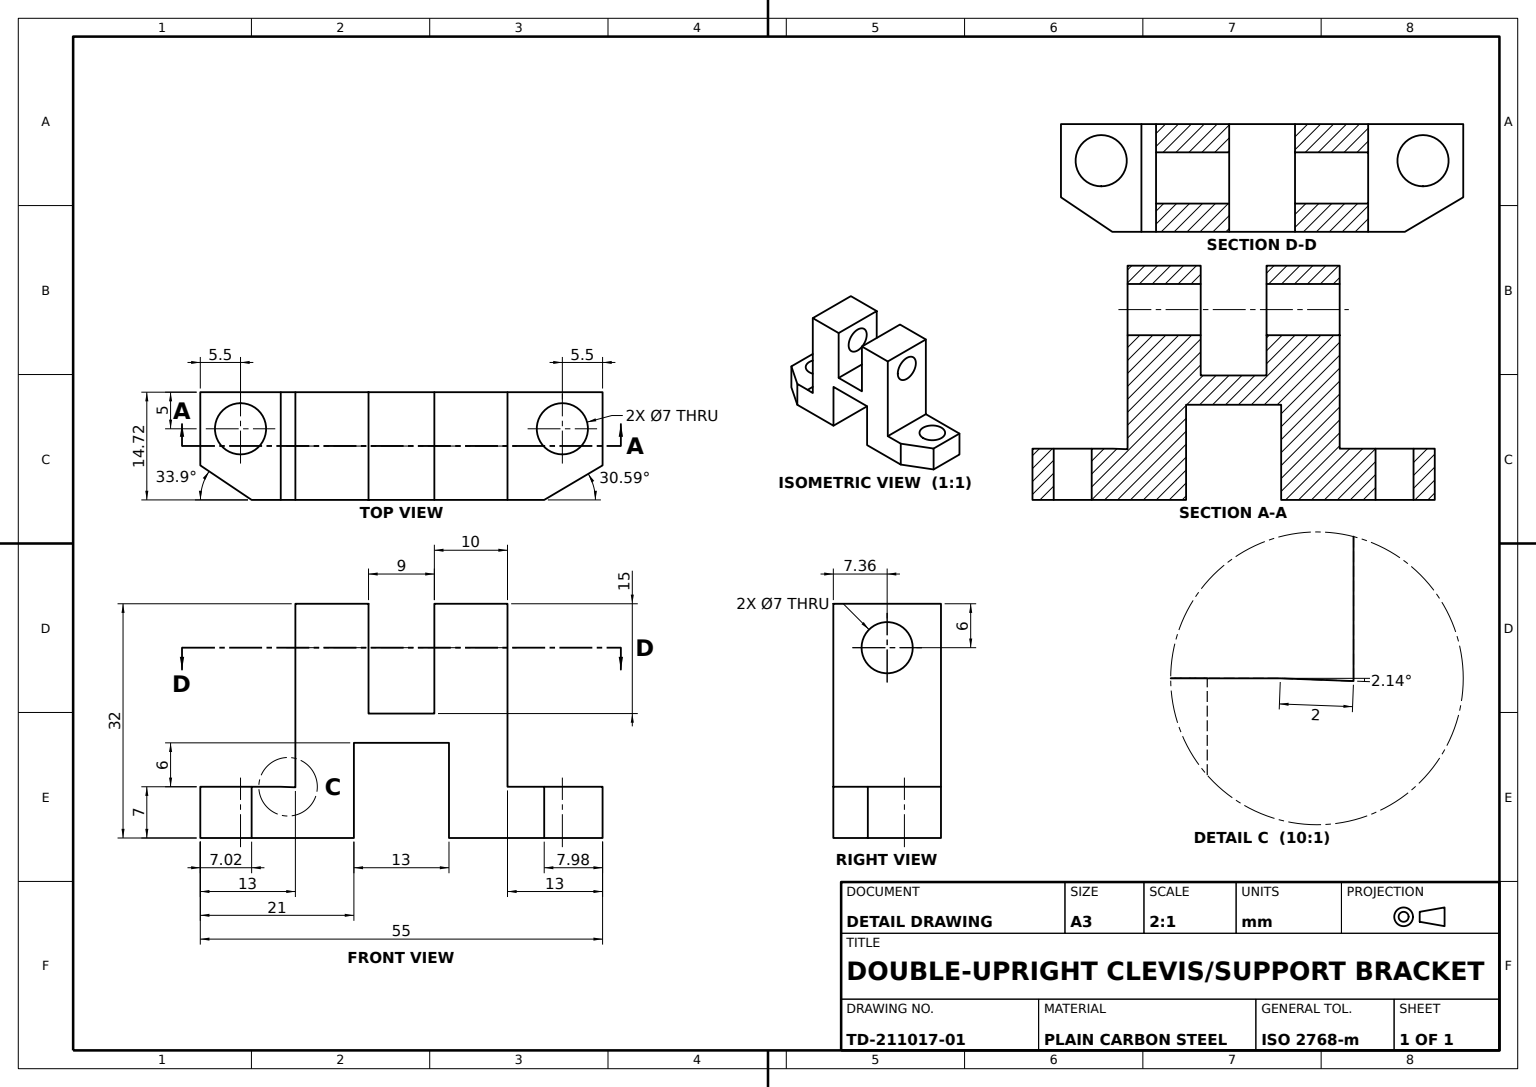
from build123d import *

# Parameters (mm, degrees)
BASE_PLATE_55X7_DEPTH         = 3.5
FRONT_NOTCH_SKETCH_W          = 13
FRONT_NOTCH_SKETCH_H          = 9.412383513
FRONT_NOTCH_13X6_5_DEPTH      = 32.38621781
UPRIGHT_A_SKETCH_W            = 10
UPRIGHT_A_SKETCH_H            = 32
UPRIGHT_A_10X32_DEPTH         = 14.717156
UPRIGHT_B_SKETCH_W            = 10
UPRIGHT_B_SKETCH_H            = 32
UPRIGHT_B_10X32_DEPTH         = 14.717156
UPRIGHT_A_HOLE_SKETCH_R       = 3.5
UPRIGHT_A_HOLE_DEPTH          = 39.016443898
INFILL_BOSS_SKETCH_W          = 13
INFILL_BOSS_SKETCH_H          = 32
INFILL_BOSS_DEPTH             = 14.717156
REAR_NOTCH_SKETCH_W           = 13
REAR_NOTCH_SKETCH_H           = 13
REAR_NOTCH_13X6_5_DEPTH       = 43.250380835
SLOT_CUT_SKETCH_W             = 9
SLOT_CUT_SKETCH_H             = 15
SLOT_CUT_DEPTH                = 43.250380835
UPRIGHT_B_HOLE_SKETCH_R       = 3.5
UPRIGHT_B_HOLE_DEPTH          = 54.030651577
FLANGE_PROFILE_CUT_A_SKETCH_W = 2
FLANGE_PROFILE_CUT_A_SKETCH_H = 25
FLANGE_PROFILE_CUT_A_DEPTH    = 43.250380835
FLANGE_PROFILE_CUT_B_DEPTH    = 43.250380835


with BuildPart() as part:
    # Base Plate Sketch → Base Plate 55x7 (new, symmetric)
    with BuildSketch(Plane(origin=(0, 0, 0), x_dir=(1, 0, 0), z_dir=(0, 1, 0))):
        Polygon((-20.480974443, -6.717155582), (19.519025557, -6.717155582), (27.5, -2), (27.5, 8), (-27.5, 8), (-27.5, -2), align=None)
    extrude(amount=BASE_PLATE_55X7_DEPTH, both=True)

    # Front Notch Sketch → Front Notch 13x6.5 (cut, through all)
    with BuildSketch(Plane.XY.offset(6.717155582)):
        with Locations((0, -0.276834809)):
            Rectangle(FRONT_NOTCH_SKETCH_W, FRONT_NOTCH_SKETCH_H)
    extrude(amount=-FRONT_NOTCH_13X6_5_DEPTH, mode=Mode.SUBTRACT)


with BuildPart() as front_notch_13x6_5_piece_1:
    # of the separate pieces the step leaves, piece 1, a body of its own (front_notch_13x6_5_pieces)
    add(part.part.solids().sort_by_distance((-20.480974443, 3.5, 6.717155582))[0])

    # Upright A Sketch → Upright A 10x32 (add)
    with BuildSketch(Plane.XY.offset(6.717155582)):
        with Locations((-11.5, 12.5)):
            Rectangle(UPRIGHT_A_SKETCH_W, UPRIGHT_A_SKETCH_H)
    extrude(amount=-UPRIGHT_A_10X32_DEPTH)


with BuildPart() as front_notch_13x6_5_piece_2:
    # of the separate pieces the step leaves, piece 2, a body of its own (front_notch_13x6_5_pieces)
    add(part.part.solids().sort_by_distance((6.5, 3.5, 6.717155582))[0])

    # Upright B Sketch → Upright B 10x32 (add)
    with BuildSketch(Plane.XY.offset(6.717155582)):
        with Locations((11.5, 12.5)):
            Rectangle(UPRIGHT_B_SKETCH_W, UPRIGHT_B_SKETCH_H)
    extrude(amount=-UPRIGHT_B_10X32_DEPTH)


with BuildPart() as upright_a_hole_tool:
    # Upright A Hole Sketch → Upright A Hole (new, through all)
    with BuildSketch(Plane(origin=(0, 3.5, 0), x_dir=(1, 0, 0), z_dir=(0, 1, 0))):
        with Locations(Location((-22, 3, 0), (0, 0, 270))):
            Circle(UPRIGHT_A_HOLE_SKETCH_R)
        with Locations(Location((22, 3, 0), (0, 0, 270))):
            Circle(UPRIGHT_A_HOLE_SKETCH_R)
    extrude(amount=-UPRIGHT_A_HOLE_DEPTH)


with BuildPart() as front_notch_13x6_5_piece_1_1:
    add(front_notch_13x6_5_piece_1.part)

    # Upright A Hole: cut by upright_a_hole_tool
    add(upright_a_hole_tool.part, mode=Mode.SUBTRACT)



with BuildPart() as front_notch_13x6_5_piece_2_1:
    add(front_notch_13x6_5_piece_2.part)

    # Upright A Hole: cut by upright_a_hole_tool
    add(upright_a_hole_tool.part, mode=Mode.SUBTRACT)


with BuildPart() as front_notch_13x6_5_piece_1_2:
    add(front_notch_13x6_5_piece_1_1.part)

    add(front_notch_13x6_5_piece_2_1.part)  # Infill Boss merges Front Notch 13x6.5 piece 2
    # Infill Boss Sketch → Infill Boss (add, through all)
    with BuildSketch(Plane.XY.offset(6.717155582)):
        with Locations((0, 12.5)):
            Rectangle(INFILL_BOSS_SKETCH_W, INFILL_BOSS_SKETCH_H)
    extrude(amount=-INFILL_BOSS_DEPTH)

    # Rear Notch Sketch → Rear Notch 13x6.5 (cut, through all)
    with BuildSketch(Plane.XY.offset(6.717155582)):
        with Locations((0, 3)):
            Rectangle(REAR_NOTCH_SKETCH_W, REAR_NOTCH_SKETCH_H)
    extrude(amount=-REAR_NOTCH_13X6_5_DEPTH, mode=Mode.SUBTRACT)

    # Slot Cut Sketch → Slot Cut (cut, through all)
    with BuildSketch(Plane.XY.offset(6.717155582)):
        with Locations((0, 21)):
            Rectangle(SLOT_CUT_SKETCH_W, SLOT_CUT_SKETCH_H)
    extrude(amount=-SLOT_CUT_DEPTH, mode=Mode.SUBTRACT)

    # Upright B Hole Sketch → Upright B Hole (cut, through all)
    with BuildSketch(Plane(origin=(16.5, 0, 0), x_dir=(0, 0, -1), z_dir=(1, 0, 0))):
        with Locations((0.641422209, 22.5)):
            Circle(UPRIGHT_B_HOLE_SKETCH_R)
    extrude(amount=-UPRIGHT_B_HOLE_DEPTH, mode=Mode.SUBTRACT)

    # Flange Profile Cut A Sketch → Flange Profile Cut A (cut, through all)
    with BuildSketch(Plane.XY.offset(6.717155582)):
        with Locations((15.5, 16)):
            Rectangle(FLANGE_PROFILE_CUT_A_SKETCH_W, FLANGE_PROFILE_CUT_A_SKETCH_H)
    extrude(amount=-FLANGE_PROFILE_CUT_A_DEPTH, mode=Mode.SUBTRACT)

    # Flange Profile Cut B Sketch → Flange Profile Cut B (cut, through all)
    with BuildSketch(Plane.XY.offset(6.717155582)):
        Polygon((-14.5, 3.425354954), (-14.5, 28.5), (-16.5, 28.5), (-16.5, 3.5), align=None)
    extrude(amount=-FLANGE_PROFILE_CUT_B_DEPTH, mode=Mode.SUBTRACT)


solid = front_notch_13x6_5_piece_1_2.part
